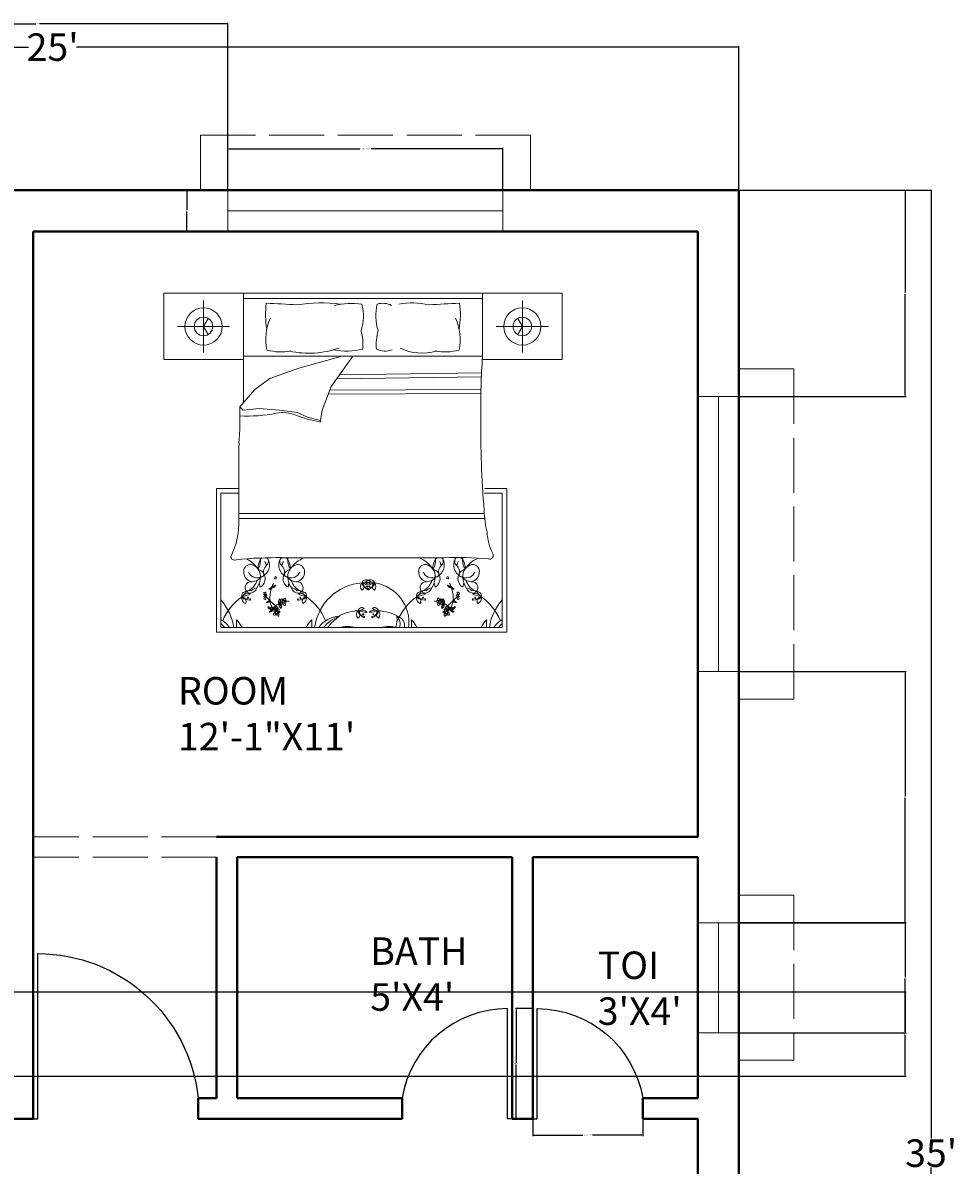
# Model space of a CAD drawing. Units: inches. Extents: x -22 to 362, y -469 to 42.
# Tile 6 of 6: x 158 to 362, y -207 to 42. Entities that reach past the tile are written whole.
import ezdxf

# ---------------------------------------------------------------- set-up
doc = ezdxf.new("R2010")
doc.units = ezdxf.units.IN
doc.header["$MEASUREMENT"] = 0
doc.linetypes.add('ACAD_ISO02W100', pattern=[15, 12, -3])
for name, color, linetype, lineweight in [('A-ANNO-DIMS', 2, 'Continuous', 18), ('A-AREA-IDEN', 7, 'Continuous', 25), ('A-DOOR', 3, 'Continuous', 25), ('A-FURN', 8, 'Continuous', 18), ('A-GLAZ', 4, 'Continuous', 20), ('A-ROOF-OVHD', 8, 'ACAD_ISO02W100', 18), ('A-WALL', 7, 'Continuous', 40), ('A-WALL-OVHD', 7, 'ACAD_ISO02W100', 18)]:
    doc.layers.add(name, color=color, linetype=linetype, lineweight=lineweight)
doc.styles.get("Standard").update_dxf_attribs({"font": 'arial.ttf'})
doc.dimstyles.get("Standard").update_dxf_attribs({"dimtxt": 0.18, "dimasz": 0.18, "dimexe": 0.18, "dimexo": 0.0625, "dimgap": 0.09, "dimtad": 0, "dimtih": 1, "dimtoh": 1, "dimdec": 0, "dimzin": 0, "dimdsep": 46, "dimlunit": 3, "dimtxsty": 'Standard', "dimcen": 0.09, "dimadec": 0, "dimazin": 0, "dimtfac": 1, "dimtdec": 0, "dimtofl": 0, "dimtmove": 0, "dimatfit": 3, "dimfxl": 1, "dimtolj": 1, "dimtzin": 0, "dimarcsym": 0})

# ---------------------------------------------------------------- blocks, each defined once
blk = doc.blocks.new('*D5')
at = {"layer": 'A-ANNO-DIMS', "color": 0, "lineweight": -2, "transparency": 16777216}
for p, q in [((15.01, 5.76), (15.01, 37.04)), ((15.19, 36.86), (159.53, 36.86)), ((314.33, 36.86), (169.99, 36.86)), ((314.51, 5.76), (314.51, 37.04))]:
    blk.add_line(p, q, dxfattribs=at)
at = {"layer": 'A-ANNO-DIMS', "color": 0, "transparency": 16777216}
for points in [[(15.19, 36.89), (15.19, 36.83), (15.01, 36.86)], [(314.33, 36.89), (314.33, 36.83), (314.51, 36.86)]]:
    blk.add_solid(points, dxfattribs=at)
at = {"layer": 'Defpoints', "color": 0, "transparency": 16777216}
for p in [(314.51, 36.86), (15.01, 5.69), (314.51, 5.69)]:
    blk.add_point(p, dxfattribs=at)
at = {"layer": 'A-ANNO-DIMS', "color": 0, "transparency": 16777216, "insert": (164.76, 36.86), "char_height": 6, "attachment_point": 5}
blk.add_mtext("\\A1;25'", dxfattribs=at)
blk = doc.blocks.new('*D6')
at = {"layer": 'A-ANNO-DIMS', "color": 0, "lineweight": -2, "transparency": 16777216}
for p, q in [((314.57, 5.69), (356.62, 5.69)), ((356.44, 5.51), (356.44, -201.15)), ((356.44, -414.13), (356.44, -207.46)), ((314.57, -414.31), (356.62, -414.31))]:
    blk.add_line(p, q, dxfattribs=at)
at = {"layer": 'A-ANNO-DIMS', "color": 0, "transparency": 16777216}
for points in [[(356.41, 5.51), (356.47, 5.51), (356.44, 5.69)], [(356.41, -414.13), (356.47, -414.13), (356.44, -414.31)]]:
    blk.add_solid(points, dxfattribs=at)
at = {"layer": 'Defpoints', "color": 0, "transparency": 16777216}
for p in [(314.51, 5.69), (314.51, -414.31), (356.44, -414.31)]:
    blk.add_point(p, dxfattribs=at)
at = {"layer": 'A-ANNO-DIMS', "color": 0, "transparency": 16777216, "insert": (356.44, -204.31), "char_height": 6, "attachment_point": 5}
blk.add_mtext("\\A1;35'", dxfattribs=at)
blk = doc.blocks.new('DOOR-SWING-36')
for p, q in [((-1, 0), (-1, 36)), ((0, 0), (-1, 0))]:
    blk.add_line(p, q)
blk.add_arc((-1, 0.81), 35.19, 90, 173.9744)
blk = doc.blocks.new('DOOR-SWING-24')
for p, q in [((-1, 0), (-1, 24)), ((0, 0), (-1, 0))]:
    blk.add_line(p, q)
blk.add_arc((-1, 0.69), 23.31, 90, 170.5843)
blk = doc.blocks.new('WIN-60-WALL9')
for p, q in [((0, 9), (60, 9)), ((0, 0), (0, 9)), ((60, 9), (60, 0)), ((0, 4.5), (60, 4.5)), ((60, 0), (0, 0))]:
    blk.add_line(p, q)
blk = doc.blocks.new('WINDOW-SHADE-72')
for p, q in [((12, 72), (0, 72)), ((12, 0), (12, 72)), ((0, 0), (12, 0))]:
    blk.add_line(p, q)
blk = doc.blocks.new('BED-DOUBLE-WITH-NIGHTSTANDS')
for p, q in [((0, 73.94), (86.94, 73.94)), ((8.69, 61.01), (8.69, 72.37)), ((17.39, 73.94), (17.39, 50.07)), ((69.55, 72.82), (17.39, 72.82)), ((78.25, 61.01), (78.25, 72.37)), ((14.37, 66.69), (3.01, 66.69)), ((72.57, 66.69), (83.93, 66.69)), ((17.39, 60.2), (69.55, 60.2)), ((29.46, 57.61), (38.94, 60.2)), ((41.27, 60.2), (36.51, 53.57)), ((23.13, 55.33), (29.46, 57.61)), ((19.78, 52.86), (23.13, 55.33)), ((69.29, 55.69), (37.72, 55.25)), ((69.32, 56.59), (38.37, 56.15)), ((16.61, 49.17), (19.78, 52.86)), ((36.51, 53.57), (34.57, 48.46)), ((69.24, 52.96), (36.23, 52.83)), ((69.24, 52.06), (35.89, 51.93)), ((17.31, 48.46), (16.61, 49.17)), ((20.84, 48.81), (17.31, 48.46)), ((25.24, 48.46), (20.84, 48.81)), ((29.11, 47.94), (25.24, 48.46)), ((31.4, 46.88), (29.11, 47.94)), ((34.57, 48.46), (34.22, 46.18)), ((34.22, 46.18), (31.4, 46.88)), ((11.48, 31.32), (16.39, 31.32)), ((11.48, 0), (11.48, 31.32)), ((16.39, 30.31), (12.48, 30.31)), ((12.48, 30.31), (12.48, 1.01)), ((73.85, 30.31), (70.02, 30.31)), ((70.04, 31.32), (74.86, 31.32)), ((73.85, 1.01), (73.85, 30.31)), ((74.86, 31.32), (74.86, 0)), ((69.95, 25.9), (16.39, 25.9)), ((70.03, 24.81), (16.39, 24.81)), ((61.12, 16.27), (25.82, 16.27)), ((21.05, 9.82), (20.86, 10.8)), ((27.13, 9.82), (27.32, 10.8)), ((59.21, 9.82), (59.02, 10.8)), ((65.28, 9.82), (65.48, 10.8)), ((74.86, 0), (11.48, 0)), ((12.48, 1.01), (73.85, 1.01))]:
    blk.add_line(p, q)
for points in [[(17.39, 59.45), (0, 59.45), (0, 73.94)], [(69.55, 73.94), (69.55, 59.45), (86.94, 59.45), (86.94, 73.94)], [(8.69, 66.69), (9.71, 68.45)], [(78.25, 66.69), (77.23, 68.45)], [(8.69, 66.69), (9.71, 64.94)], [(78.25, 66.69), (77.23, 64.94)]]:
    blk.add_lwpolyline(points)
for points in [[(22.38, 71.77, 0.074897), (22.49, 66.09, -0.472817)], [(43.06, 65.77, 0.14099), (43.24, 71.57, 0.235245)], [(46.78, 65.77, -0.14099), (46.6, 71.57, -0.235245)], [(64.56, 71.77, -0.074897), (64.45, 66.09, 0.472817)], [(16.43, 41.21, 0.001242), (16.39, 24.71, -0.127202), (14.64, 16.49)], [(69.92, 26.58, 0.056112), (70.55, 21.8, 0.095341), (71.78, 17.19)]]:
    blk.add_lwpolyline(points, format="xyb")
for centre, radius in [((8.69, 66.69), 4.06), ((78.25, 66.69), 4.06), ((8.69, 66.69), 2.03), ((78.25, 66.69), 2.03), ((26.07, 6.67), 0.221), ((60.26, 6.67), 0.221), ((24.62, 4.34), 0.221), ((61.71, 4.34), 0.221)]:
    blk.add_circle(centre, radius)
for centre, radius, start, end in [((70.3, 899.16), 828.77, 266.68521, 267.14978), ((34.29, 40.31), 31.53, 82.2196, 99.497), ((40.95, 56.24), 15.49, 81.5249, 103.96), ((47.79, 67.44), 4.3, 63.3437, 106.1026), ((54.24, 56.56), 15.28, 76.3427, 101.1841), ((16.64, 899.16), 828.77, 272.85022, 273.31479), ((33.46, 63.81), 11.21, 155.1316, 191.7583), ((53.48, 63.81), 11.21, 348.2417, 24.8684), ((32.81, 62.87), 10.65, 354.0129, 15.8293), ((57.02, 62.87), 10.65, 164.1707, 185.9871), ((25.48, 72.79), 11.65, 255.1039, 281.0369), ((31.62, 81.07), 20.21, 258.0397, 289.2615), ((39.8, 76.66), 15.33, 259.8617, 283.6238), ((48.38, 65.93), 4.61, 245.0183, 288.5407), ((56.43, 71.93), 11.07, 243.8761, 286.1746), ((61.46, 72.79), 11.65, 258.9631, 284.8961), ((225.41, 49.57), 156.22, 176.1, 180.9282), ((-63.11, 47.01), 79.74, 355.8294, 1.553), ((18.1, 79.95), 32.81, 267.4519, 281.3392), ((25.94, 40.84), 7.08, 66.2616, 101.3392), ((40.26, 79.03), 33.72, 250.1194, 259.3383), ((34.02, 46.1), 0.21, 268.8623, 19.7536), ((272.96, 43.89), 203.78, 179.1145, 184.8735), ((15.44, 16.54), 0.802, 183.98, 297.3412), ((24.78, -74.23), 90.51, 89.3433, 95.6887), ((15.1, 10.15), 6.58, 33.6671, 63.2997), ((23.92, 14.06), 3.35, 145.785, 184.7304), ((17.52, 15.63), 3.6, 328.8218, 9.1554), ((21.98, 15.31), 1.05, 120.0293, 142.325), ((20.31, 14.69), 2.77, 289.2822, 29.1751), ((19.89, 14.19), 2.5, 7.436, 29.9149), ((21.54, 15.52), 1.3, 311.5653, 23.8354), ((21.98, 15.31), 1.05, 44.4517, 63.558), ((27.87, 14.69), 2.77, 150.8249, 250.7178), ((26.64, 15.52), 1.3, 156.1646, 228.4347), ((26.2, 15.31), 1.05, 113.229, 135.5483), ((28.29, 14.19), 2.5, 150.0851, 172.564), ((26.2, 15.31), 1.05, 37.675, 66.7144), ((24.25, 14.06), 3.35, 355.2696, 34.215), ((30.66, 15.63), 3.6, 169.7133, 211.1782), ((33.07, 10.15), 6.58, 111.4941, 146.3329), ((53.26, 10.15), 6.58, 33.6671, 68.5059), ((62.08, 14.06), 3.35, 145.785, 184.7304), ((55.68, 15.63), 3.6, 328.8218, 10.2867), ((60.14, 15.31), 1.05, 113.2856, 142.325), ((58.46, 14.69), 2.77, 289.2822, 29.1751), ((58.05, 14.19), 2.5, 7.436, 29.9149), ((60.14, 15.31), 1.05, 44.4517, 66.7144), ((59.69, 15.52), 1.3, 311.5653, 23.8354), ((63.78, -68.29), 84.6, 85.2402, 91.8035), ((66.03, 14.69), 2.77, 150.8249, 250.7178), ((64.8, 15.52), 1.3, 156.1646, 228.4347), ((64.35, 15.31), 1.05, 106.6343, 135.5483), ((66.44, 14.19), 2.5, 150.0851, 172.564), ((64.35, 15.31), 1.05, 37.675, 72.5814), ((62.41, 14.06), 3.35, 355.2696, 34.215), ((68.82, 15.63), 3.6, 169.249, 211.1782), ((71.23, 10.15), 6.58, 113.6453, 146.3329), ((71.12, 16.75), 0.792, 246.5219, 33.8264), ((19.54, 13.1), 2.08, 174.9449, 262.8857), ((18.94, 13.31), 1.47, 84.4856, 181.0538), ((20.36, 13.89), 2.02, 201.5819, 291.4221), ((18.49, 12.22), 2.61, 355.2933, 76.921), ((19.97, 11.7), 2.16, 299.9085, 73.1337), ((21.34, 12.6), 0.54, 257.3041, 15.1471), ((23.58, 13.21), 1.78, 131.5653, 195.1471), ((24.59, 13.21), 1.78, 344.8529, 48.4347), ((28.2, 11.7), 2.16, 106.8663, 240.0915), ((26.84, 12.6), 0.54, 164.8529, 282.6959), ((29.69, 12.22), 2.61, 103.079, 184.7067), ((27.82, 13.89), 2.02, 248.5779, 338.4181), ((28.64, 13.1), 2.08, 277.1143, 5.0551), ((29.24, 13.31), 1.47, 358.9462, 95.5144), ((57.7, 13.1), 2.08, 174.9449, 262.8857), ((57.09, 13.31), 1.47, 84.4856, 181.0538), ((58.51, 13.89), 2.02, 201.5819, 291.4221), ((56.64, 12.22), 2.61, 355.2933, 76.921), ((58.13, 11.7), 2.16, 299.9085, 73.1337), ((59.5, 12.6), 0.54, 257.3041, 15.1471), ((61.74, 13.21), 1.78, 131.5653, 195.1471), ((62.75, 13.21), 1.78, 344.8529, 48.4347), ((66.36, 11.7), 2.16, 106.8663, 240.0915), ((64.99, 12.6), 0.54, 164.8529, 282.6959), ((67.85, 12.22), 2.61, 103.079, 184.7067), ((65.98, 13.89), 2.02, 248.5779, 338.4181), ((66.79, 13.1), 2.08, 277.1143, 5.0551), ((67.4, 13.31), 1.47, 358.9462, 95.5144), ((19.06, 9.75), 1.3, 80.264, 250.8688), ((16.47, 12.62), 4.1, 301.2614, 341.7045), ((19.18, 13.56), 2.53, 272.3591, 324.0401), ((16.44, 12.29), 4.67, 326.2883, 356.5076), ((23.92, 14.06), 3.35, 212.7011, 216.3445), ((30.36, 7.41), 7.2, 153.0032, 159.8941), ((23.87, 9.87), 0.177, 84.3784, 186.0543), ((23.52, 11.4), 1.4, 285.5129, 293.6099), ((23.37, 11.14), 1.37, 301.164, 321.5612), ((24.43, 9.82), 0.456, 87.3579, 140.4944), ((24.34, 11.79), 0.168, 102.7051, 280.4384), ((22.26, 11.38), 2.45, 324.6898, 333.4936), ((24.32, 11.89), 0.272, 280.4384, 100.4136), ((24.25, 14.06), 3.35, 323.6555, 327.2989), ((29, 13.56), 2.53, 215.9599, 267.6409), ((31.74, 12.29), 4.67, 183.4924, 213.7117), ((31.7, 12.62), 4.1, 198.2955, 238.7386), ((29.12, 9.75), 1.3, 289.1312, 99.736), ((44.15, -0.52), 11.35, 94.4623, 172.255), ((44.2, 9.95), 1.26, 137.7873, 219.1145), ((42.77, 9.99), 0.948, 298.5391, 58.3627), ((44.17, 10.53), 0.941, 63.0274, 163.8037), ((43.21, 12.73), 1.94, 271.4585, 315.3727), ((44, 9.16), 1.79, 45.5411, 114.3101), ((45.64, 18.38), 7.94, 252.593, 267.2582), ((44.19, 10.76), 0.929, 177.7585, 283.852), ((45.98, 11.73), 2.87, 198.9159, 238.011), ((45.23, 9.16), 1.79, 65.6899, 134.4589), ((43.59, 18.38), 7.94, 272.7418, 287.407), ((44.38, 9.98), 0.123, 283.852, 219.9245), ((45.07, 10.53), 0.941, 16.1963, 116.9726), ((46.02, 12.73), 1.94, 224.6273, 268.5415), ((44.84, 10.03), 0.074, 320.1909, 256.0209), ((43.25, 11.73), 2.87, 301.989, 341.0841), ((45.04, 10.76), 0.929, 256.148, 2.2415), ((46.47, 9.99), 0.948, 121.6373, 241.4609), ((45.04, 9.95), 1.26, 320.8855, 42.2127), ((44.72, 2.1), 8.79, 352.8636, 81.8197), ((57.22, 9.75), 1.3, 80.264, 250.8688), ((54.63, 12.62), 4.1, 301.2614, 341.7045), ((57.34, 13.56), 2.53, 272.3591, 324.0401), ((54.59, 12.29), 4.67, 326.2883, 356.5076), ((62.08, 14.06), 3.35, 212.7011, 216.3445), ((62.01, 11.89), 0.272, 79.5864, 259.5616), ((62.96, 11.14), 1.37, 218.4388, 238.836), ((61.9, 9.82), 0.456, 39.5056, 92.6421), ((64.08, 11.38), 2.45, 206.5064, 215.3102), ((62, 11.79), 0.168, 259.5616, 77.2949), ((62.82, 11.4), 1.4, 246.3901, 254.4871), ((55.97, 7.41), 7.2, 20.1059, 26.9968), ((62.46, 9.87), 0.177, 353.9457, 95.6216), ((62.41, 14.06), 3.35, 323.6555, 327.2989), ((67.16, 13.56), 2.53, 215.9599, 267.6409), ((69.9, 12.29), 4.67, 183.4924, 213.7117), ((69.86, 12.62), 4.1, 198.2955, 238.7386), ((67.27, 9.75), 1.3, 289.1312, 99.736), ((23.45, -1.64), 11.35, 124.3865, 158.5908), ((18.27, 7.46), 1.26, 167.7115, 249.0387), ((17.96, 7.95), 0.941, 92.9516, 193.728), ((16.03, 9.38), 1.94, 301.3827, 345.2969), ((18.5, 6.68), 1.79, 75.4653, 144.2343), ((15.32, 15.48), 7.94, 282.5173, 297.1824), ((17.01, 6.78), 0.948, 328.4633, 88.2869), ((18.93, 9.89), 2.87, 228.8402, 267.9352), ((17.86, 8.16), 0.929, 207.6827, 313.7762), ((18.79, 8.34), 0.8, 63.9755, 143.2681), ((18.42, 7.57), 0.123, 313.7762, 249.7183), ((18.75, 10.14), 1.63, 265.969, 344.3045), ((20.5, 7.98), 1.74, 96.1662, 141.5825), ((22.09, 8.33), 0.369, 101.5637, 142.6358), ((21.78, 7.99), 0.221, 273.2768, 86.7232), ((22.04, 8.2), 0.211, 91.1081, 181.8675), ((22.48, 8.06), 0.672, 203.4276, 227.6104), ((22.26, 7.77), 0.458, 80.3487, 133.6538), ((22.18, 8.15), 0.362, 229.7889, 317.6792), ((21.79, 8.62), 0.532, 288.7263, 352.5032), ((21.77, 7.38), 0.515, 355.053, 68.3618), ((22.18, 7.3), 0.725, 83.0852, 105.7171), ((22.15, 8.59), 0.171, 345.2356, 144.9248), ((17.16, 1.28), 8.25, 43.1541, 52.0459), ((22.31, 8.03), 0.191, 317.6792, 80.3487), ((23.38, 9.2), 0.456, 101.3256, 154.4621), ((22.72, 10.74), 1.37, 280.2588, 300.656), ((23.04, 11.84), 2.45, 268.3264, 277.1302), ((30.36, 7.41), 7.2, 163.5842, 183.8277), ((22.42, 10.74), 1.4, 308.2101, 316.3071), ((23.28, 9.82), 0.417, 278.3432, 4.2869), ((23.05, 10.19), 0.729, 300.656, 332.6341), ((23.6, 9.71), 0.177, 55.7657, 157.4417), ((23.71, 10.58), 0.729, 269.1859, 301.164), ((23.92, 10.21), 0.417, 237.5332, 323.4768), ((27.67, 7.98), 1.74, 38.4175, 83.8338), ((29.43, 10.14), 1.63, 195.6955, 274.031), ((29.38, 8.34), 0.8, 36.7319, 116.0245), ((29.68, 6.68), 1.79, 35.7657, 104.5347), ((32.86, 15.48), 7.94, 242.8176, 257.4827), ((29.24, 9.89), 2.87, 272.0648, 311.1598), ((30.31, 8.16), 0.929, 226.2238, 332.3173), ((29.77, 7.62), 0.074, 290.2667, 226.2271), ((31.16, 6.78), 0.948, 91.7131, 211.5367), ((30.22, 7.95), 0.941, 346.272, 87.0484), ((32.14, 9.38), 1.94, 194.7031, 238.6173), ((29.9, 7.46), 1.26, 290.9613, 12.2885), ((24.72, -1.64), 11.35, 21.4092, 55.6135), ((44.53, 9.41), 0.141, 238.011, 71.5592), ((44.56, 9.48), 0.0685, 71.5592, 188.0167), ((44.7, 9.41), 0.141, 108.4408, 301.989), ((44.68, 9.48), 0.0685, 351.9833, 108.4408), ((61.61, -1.64), 11.35, 124.3865, 158.5908), ((56.11, 7.95), 0.941, 92.9516, 193.728), ((56.43, 7.46), 1.26, 167.7115, 249.0387), ((54.19, 9.38), 1.94, 301.3827, 345.2969), ((56.66, 6.68), 1.79, 75.4653, 144.2343), ((53.48, 15.48), 7.94, 282.5173, 297.1824), ((56.02, 8.16), 0.929, 207.6827, 313.7762), ((57.09, 9.89), 2.87, 228.8402, 267.9352), ((55.17, 6.78), 0.948, 328.4633, 88.2869), ((56.95, 8.34), 0.8, 63.9755, 143.2681), ((56.58, 7.57), 0.123, 313.7762, 249.7183), ((56.91, 10.14), 1.63, 265.969, 344.3045), ((58.66, 7.98), 1.74, 96.1662, 141.5825), ((62.41, 10.21), 0.417, 216.5232, 302.4668), ((62.63, 10.58), 0.729, 238.836, 270.8141), ((62.74, 9.71), 0.177, 22.5583, 124.2343), ((63.05, 9.82), 0.417, 175.7131, 261.6568), ((63.28, 10.19), 0.729, 207.3659, 239.344), ((55.97, 7.41), 7.2, 356.1723, 16.4158), ((63.91, 10.74), 1.4, 223.6929, 231.7899), ((63.61, 10.74), 1.37, 239.344, 259.7412), ((63.3, 11.84), 2.45, 262.8698, 271.6736), ((62.96, 9.2), 0.456, 25.5379, 78.6744), ((69.18, 1.28), 8.25, 127.9541, 136.8459), ((64.03, 8.03), 0.191, 99.6513, 222.3208), ((64.15, 8.15), 0.362, 222.3208, 310.2111), ((64.07, 7.77), 0.458, 46.3462, 99.6513), ((64.18, 8.59), 0.171, 35.0752, 194.7644), ((64.54, 8.62), 0.532, 187.4968, 251.2737), ((64.56, 7.38), 0.515, 111.6382, 184.947), ((64.16, 7.3), 0.725, 74.2829, 96.9148), ((64.29, 8.2), 0.211, 358.1325, 88.8919), ((63.86, 8.06), 0.672, 312.3896, 336.5724), ((64.25, 8.33), 0.369, 37.3642, 78.4363), ((64.55, 7.99), 0.221, 93.2768, 266.7232), ((67.59, 10.14), 1.63, 195.6955, 274.031), ((65.83, 7.98), 1.74, 38.4175, 83.8338), ((67.54, 8.34), 0.8, 36.7319, 116.0245), ((67.84, 6.68), 1.79, 35.7657, 104.5347), ((71.01, 15.48), 7.94, 242.8176, 257.4827), ((67.4, 9.89), 2.87, 272.0648, 311.1598), ((68.47, 8.16), 0.929, 226.2238, 332.3173), ((67.93, 7.62), 0.074, 290.2667, 226.2271), ((69.32, 6.78), 0.948, 91.7131, 211.5367), ((70.3, 9.38), 1.94, 194.7031, 238.6173), ((68.38, 7.95), 0.941, 346.272, 87.0484), ((68.06, 7.46), 1.26, 290.9613, 12.2885), ((62.88, -1.64), 11.35, 21.4092, 55.6135), ((4.03, -0.52), 11.35, 7.745, 41.8856), ((18.82, 7.23), 0.0685, 101.4834, 217.9409), ((18.83, 7.16), 0.141, 267.9352, 101.4834), ((22.08, 7.58), 0.366, 217.7621, 259.0403), ((22.12, 7.35), 0.17, 232.4737, 355.053), ((22.86, 6.27), 0.456, 101.3256, 154.4621), ((22.2, 7.82), 1.37, 280.2588, 300.656), ((22.52, 8.92), 2.45, 268.3264, 277.1302), ((21.91, 7.82), 1.4, 308.2101, 316.3071), ((23.01, 5.47), 0.247, 146.8636, 236.9021), ((26.5, 10.92), 6.47, 235.1882, 238.8844), ((23.44, 5.83), 0.669, 199.4799, 267.6828), ((22.76, 6.9), 0.417, 278.3432, 4.2869), ((23.36, 5.57), 0.576, 212.8155, 277.3992), ((22.53, 7.26), 0.729, 300.656, 332.6341), ((23.08, 6.78), 0.177, 55.7657, 157.4417), ((23.29, 5.6), 0.256, 238.8844, 314.2646), ((26.78, 7.23), 3.61, 184.756, 209.2041), ((31.97, 14.91), 11.88, 222.2412, 232.1744), ((23.23, 5.02), 0.576, 280.3057, 17.1958), ((23.18, 4.96), 0.256, 306.3746, 21.7548), ((23.6, 5.13), 0.193, 19.3605, 201.7548), ((23.6, 5.27), 0.193, 311.8703, 134.2646), ((27.23, 3.52), 3.86, 153.7819, 158.2913), ((24.16, 6.15), 1.01, 247.2305, 319.0635), ((23.83, 5.81), 0.594, 264.4544, 310.6188), ((26.78, 7.23), 3.61, 214.0033, 222.4917), ((24.27, 5.57), 0.613, 218.3208, 298.8162), ((27.15, 2.43), 4.33, 120.544, 139.818), ((24.68, 4.82), 0.714, 70.0041, 130.6188), ((24.22, 5.69), 0.733, 297.7043, 344.3516), ((24.93, 4.68), 0.369, 101.5637, 176.365), ((25, 4.94), 0.171, 345.2356, 144.9248), ((24.38, 7), 1.01, 304.5369, 16.3699), ((24.92, 6.78), 0.613, 272.8499, 356.1226), ((24.48, 6.54), 0.594, 321.7607, 7.9252), ((24.61, 5.68), 0.594, 8.7227, 54.8872), ((24.64, 5.21), 1.01, 0.278, 72.111), ((25.78, 6.72), 0.714, 127.3105, 187.9252), ((25.09, 5.58), 0.613, 20.5253, 88.5375), ((25.9, 5.88), 0.714, 188.7227, 249.3375), ((24.8, 6.8), 0.733, 355.0106, 41.658), ((25.61, 6.26), 0.219, 148.0499, 225.6268), ((27.15, 2.43), 4.33, 113.0501, 113.8477), ((26.01, 6), 0.698, 104.7558, 148.0499), ((25.62, 6.5), 0.437, 247.4086, 351.4386), ((25.83, 6.98), 0.302, 126.1046, 271.4281), ((25.8, 7.06), 0.217, 353.7526, 131.7054), ((24.99, 5.52), 0.733, 334.9899, 21.6373), ((25.75, 6.48), 0.147, 262.906, 7.132), ((25.59, 6.8), 0.305, 0.0645, 61.1507), ((25.66, 7.06), 0.348, 311.8413, 355.7877), ((26.38, 7.01), 0.369, 101.5637, 176.365), ((26.37, 6.26), 0.366, 151.2196, 259.0403), ((26.33, 6.88), 0.211, 91.1081, 181.8675), ((26.77, 6.75), 0.672, 203.4276, 227.6104), ((26.56, 6.46), 0.458, 80.3487, 133.6538), ((26.47, 6.83), 0.362, 229.7889, 317.6792), ((26.08, 7.3), 0.532, 288.7263, 352.5032), ((26.07, 6.07), 0.515, 355.053, 68.3618), ((26.47, 5.98), 0.725, 83.0852, 105.7171), ((26.45, 7.28), 0.171, 345.2356, 144.9248), ((26.41, 6.04), 0.17, 232.4737, 355.053), ((26.6, 6.72), 0.191, 317.6792, 80.3487), ((27.15, 2.43), 4.33, 87.1071, 94.7585), ((29.34, 7.16), 0.141, 78.5166, 272.0648), ((29.36, 7.23), 0.0685, 322.0591, 78.5166), ((43.3, 4.45), 0.941, 63.0274, 163.8037), ((42.34, 6.65), 1.94, 271.4585, 315.3727), ((45.93, 4.45), 0.941, 16.1963, 116.9726), ((46.89, 6.65), 1.94, 224.6273, 268.5415), ((56.98, 7.23), 0.0685, 101.4834, 217.9409), ((56.99, 7.16), 0.141, 267.9352, 101.4834), ((59.19, 2.43), 4.33, 85.2415, 92.8929), ((59.73, 6.72), 0.191, 99.6513, 222.3208), ((59.86, 6.83), 0.362, 222.3208, 310.2111), ((59.78, 6.46), 0.458, 46.3462, 99.6513), ((59.89, 7.28), 0.171, 35.0752, 194.7644), ((60.25, 7.3), 0.532, 187.4968, 251.2737), ((60.27, 6.07), 0.515, 111.6382, 184.947), ((59.93, 6.04), 0.17, 184.947, 307.5263), ((59.87, 5.98), 0.725, 74.2829, 96.9148), ((60, 6.88), 0.211, 358.1325, 88.8919), ((59.56, 6.75), 0.672, 312.3896, 336.5724), ((59.95, 7.01), 0.369, 3.635, 78.4363), ((59.96, 6.26), 0.366, 280.9597, 28.7804), ((60.71, 6.5), 0.437, 188.5614, 292.5914), ((60.54, 7.06), 0.217, 48.2946, 186.2474), ((60.67, 7.06), 0.348, 184.2123, 228.1587), ((60.74, 6.8), 0.305, 118.8493, 179.9355), ((60.59, 6.48), 0.147, 172.868, 277.094), ((60.51, 6.98), 0.302, 268.5719, 53.8954), ((60.32, 6), 0.698, 31.9501, 75.2442), ((61.35, 5.52), 0.733, 158.3627, 205.0101), ((61.24, 5.58), 0.613, 91.4625, 159.4747), ((61.69, 5.21), 1.01, 107.889, 179.722), ((60.43, 5.88), 0.714, 290.6625, 351.2773), ((61.54, 6.8), 0.733, 138.342, 184.9894), ((61.42, 6.78), 0.613, 183.8774, 267.1501), ((59.19, 2.43), 4.33, 66.1523, 66.9499), ((60.73, 6.26), 0.219, 314.3732, 31.9501), ((61.96, 7), 1.01, 163.6301, 235.4631), ((60.55, 6.72), 0.714, 352.0748, 52.6895), ((61.73, 5.68), 0.594, 125.1128, 171.2773), ((61.34, 4.94), 0.171, 35.0752, 194.7644), ((61.85, 6.54), 0.594, 172.0748, 218.2393), ((59.19, 2.43), 4.33, 40.182, 59.456), ((61.65, 4.82), 0.714, 49.3812, 109.9959), ((62.17, 6.15), 1.01, 220.9365, 292.7695), ((62.11, 5.69), 0.733, 195.6484, 242.2957), ((61.4, 4.68), 0.369, 3.635, 78.4363), ((54.36, 14.91), 11.88, 307.8256, 317.7588), ((62.07, 5.57), 0.613, 241.1838, 321.6792), ((62.5, 5.81), 0.594, 229.3812, 275.5456), ((59.56, 7.23), 3.61, 317.5083, 325.9967), ((63.1, 5.02), 0.576, 162.8042, 259.6943), ((62.73, 5.27), 0.193, 45.7354, 228.1297), ((62.73, 5.13), 0.193, 338.2452, 160.6395), ((59.1, 3.52), 3.86, 21.7087, 26.2181), ((59.56, 7.23), 3.61, 330.7959, 355.244), ((63.04, 5.6), 0.256, 225.7354, 301.1156), ((63.15, 4.96), 0.256, 158.2452, 233.6254), ((62.97, 5.57), 0.576, 262.6008, 327.1845), ((62.9, 5.83), 0.669, 272.3172, 340.5201), ((63.25, 6.78), 0.177, 22.5583, 124.2343), ((63.57, 6.9), 0.417, 175.7131, 261.6568), ((63.8, 7.26), 0.729, 207.3659, 239.344), ((59.83, 10.92), 6.47, 301.1156, 304.8118), ((64.43, 7.82), 1.4, 223.6929, 231.7899), ((64.13, 7.82), 1.37, 239.344, 259.7412), ((63.32, 5.47), 0.247, 303.0979, 33.1364), ((63.81, 8.92), 2.45, 262.8698, 271.6736), ((63.47, 6.27), 0.456, 25.5379, 78.6744), ((64.22, 7.35), 0.17, 184.947, 307.5263), ((64.25, 7.58), 0.366, 280.9597, 322.2379), ((67.5, 7.16), 0.141, 78.5166, 272.0648), ((67.51, 7.23), 0.0685, 322.0591, 78.5166), ((82.3, -0.52), 11.35, 138.1144, 172.255), ((9.73, -2.04), 5.53, 33.4617, 60.1116), ((12.82, -0.76), 4.62, 22.5547, 48.9546), ((0.18, 1.72), 15.71, 357.4081, 3.6519), ((23.03, 5.19), 0.669, 266.9701, 338.2913), ((19.5, 9.97), 6.47, 302.6784, 306.3746), ((23.2, 4.66), 0.247, 214.3538, 304.3923), ((24.16, 3.92), 0.219, 148.0499, 225.6268), ((24.57, 3.67), 0.698, 104.7558, 148.0499), ((24.17, 4.17), 0.437, 247.4086, 351.4386), ((24.38, 4.65), 0.302, 126.1046, 271.4281), ((24.35, 4.73), 0.217, 353.7526, 131.7054), ((24.3, 4.15), 0.147, 262.906, 7.132), ((24.14, 4.47), 0.305, 0.0645, 61.1507), ((24.22, 4.73), 0.348, 311.8413, 355.7877), ((24.93, 3.93), 0.366, 151.2196, 259.0403), ((24.88, 4.55), 0.211, 91.1081, 181.8675), ((25.32, 4.41), 0.672, 203.4276, 227.6104), ((25.11, 4.12), 0.458, 80.3487, 133.6538), ((25.03, 4.5), 0.362, 229.7889, 317.6792), ((24.63, 4.97), 0.532, 288.7263, 352.5032), ((24.62, 3.73), 0.515, 355.053, 68.3618), ((25.02, 3.65), 0.725, 83.0852, 105.7171), ((24.96, 3.7), 0.17, 232.4737, 355.053), ((25.15, 4.39), 0.191, 317.6792, 80.3487), ((35.35, -0.76), 4.62, 131.0454, 157.4453), ((48, 1.72), 15.71, 176.3481, 182.5919), ((38.45, -2.04), 5.53, 91.272, 146.5383), ((40.44, -3.07), 6.89, 107.8504, 143.6964), ((44.06, -5.01), 10.25, 124.0123, 144.053), ((43.28, -6.6), 11.35, 94.4623, 117.4146), ((43.33, 3.87), 1.26, 137.7873, 219.1145), ((41.9, 3.91), 0.948, 298.5391, 58.3627), ((43.13, 3.08), 1.79, 45.5411, 114.3101), ((45.11, 5.65), 2.87, 198.9159, 238.011), ((44.77, 12.29), 7.94, 252.593, 267.2582), ((43.32, 4.68), 0.929, 177.7585, 283.852), ((43.51, 3.9), 0.123, 283.852, 219.9245), ((43.66, 3.33), 0.141, 238.011, 71.5592), ((43.69, 3.4), 0.0685, 71.5592, 188.0167), ((46.1, 3.08), 1.79, 65.6899, 134.4589), ((44.46, 12.29), 7.94, 272.7418, 287.407), ((45.57, 3.33), 0.141, 108.4408, 301.989), ((45.55, 3.4), 0.0685, 351.9833, 108.4408), ((45.71, 3.94), 0.074, 320.1909, 256.0209), ((44.12, 5.65), 2.87, 301.989, 341.0841), ((45.91, 4.68), 0.929, 256.148, 2.2415), ((47.34, 3.91), 0.948, 121.6373, 241.4609), ((45.91, 3.87), 1.26, 320.8855, 42.2127), ((45.95, -6.6), 11.35, 62.5854, 85.5377), ((45.85, 2.9), 5.08, 338.117, 6.6195), ((50.52, 1.49), 2.04, 346.3898, 79.0739), ((48.99, 1.77), 2.58, 342.8609, 41.9049), ((38.34, 1.72), 15.71, 357.4081, 3.6519), ((50.98, -0.76), 4.62, 22.5547, 48.9546), ((61.18, 4.39), 0.191, 99.6513, 222.3208), ((61.31, 4.5), 0.362, 222.3208, 310.2111), ((61.23, 4.12), 0.458, 46.3462, 99.6513), ((61.7, 4.97), 0.532, 187.4968, 251.2737), ((61.72, 3.73), 0.515, 111.6382, 184.947), ((61.37, 3.7), 0.17, 184.947, 307.5263), ((61.31, 3.65), 0.725, 74.2829, 96.9148), ((61.45, 4.55), 0.211, 358.1325, 88.8919), ((61.01, 4.41), 0.672, 312.3896, 336.5724), ((61.41, 3.93), 0.366, 280.9597, 28.7804), ((62.16, 4.17), 0.437, 188.5614, 292.5914), ((61.99, 4.73), 0.217, 48.2946, 186.2474), ((62.12, 4.73), 0.348, 184.2123, 228.1587), ((62.19, 4.47), 0.305, 118.8493, 179.9355), ((62.04, 4.15), 0.147, 172.868, 277.094), ((61.95, 4.65), 0.302, 268.5719, 53.8954), ((61.77, 3.67), 0.698, 31.9501, 75.2442), ((62.17, 3.92), 0.219, 314.3732, 31.9501), ((63.31, 5.19), 0.669, 201.7087, 273.0299), ((66.83, 9.97), 6.47, 233.6254, 237.3216), ((63.14, 4.66), 0.247, 235.6077, 325.6462), ((73.51, -0.76), 4.62, 131.0454, 157.4453), ((86.15, 1.72), 15.71, 176.3481, 182.5919), ((76.61, -2.04), 5.53, 119.8884, 146.5383), ((7.74, -3.07), 6.89, 36.3036, 46.4814), ((40.1, -4.96), 6.24, 73.5431, 107.0202), ((42.58, -8.18), 9.23, 94.3787, 95.6357), ((47.44, -14.5), 16.5, 109.7217, 109.9028), ((49.13, -4.96), 6.24, 72.9798, 106.4569), ((46.66, -8.18), 9.23, 84.3643, 85.6213), ((41.79, -14.5), 16.5, 70.0972, 70.2783), ((78.6, -3.07), 6.89, 133.5186, 143.6964)]:
    blk.add_arc(centre, radius, start, end)
blk = doc.blocks.new('*D14')
at = {"layer": 'A-ANNO-DIMS', "color": 0, "lineweight": -2, "transparency": 16777216}
for p, q in [((203.01, 5.76), (203.01, 14.87)), ((203.19, 14.69), (231.78, 14.69)), ((262.83, 14.69), (234.24, 14.69)), ((263.01, 5.76), (263.01, 14.87))]:
    blk.add_line(p, q, dxfattribs=at)
at = {"layer": 'A-ANNO-DIMS', "color": 0, "transparency": 16777216}
for points in [[(203.19, 14.72), (203.19, 14.66), (203.01, 14.69)], [(262.83, 14.72), (262.83, 14.66), (263.01, 14.69)]]:
    blk.add_solid(points, dxfattribs=at)
at = {"layer": 'Defpoints', "color": 0, "transparency": 16777216}
for p in [(203.01, 14.69), (203.01, 5.69), (263.01, 5.69)]:
    blk.add_point(p, dxfattribs=at)
at = {"layer": 'A-ANNO-DIMS', "color": 0, "transparency": 16777216, "insert": (233.01, 14.69), "char_height": 0.18, "attachment_point": 5}
blk.add_mtext('\\A1;WINDOW 5\'-0" TYP.', dxfattribs=at)
blk = doc.blocks.new('*D15')
at = {"layer": 'A-ANNO-DIMS', "color": 0, "lineweight": -2, "transparency": 16777216}
for p, q in [((202.95, 5.69), (193.83, 5.69)), ((194.01, 5.51), (194.01, 1.38)), ((194.01, -3.13), (194.01, 1.01)), ((202.95, -3.31), (193.83, -3.31))]:
    blk.add_line(p, q, dxfattribs=at)
at = {"layer": 'A-ANNO-DIMS', "color": 0, "transparency": 16777216}
for points in [[(193.98, 5.51), (194.04, 5.51), (194.01, 5.69)], [(193.98, -3.13), (194.04, -3.13), (194.01, -3.31)]]:
    blk.add_solid(points, dxfattribs=at)
at = {"layer": 'Defpoints', "color": 0, "transparency": 16777216}
for p in [(203.01, 5.69), (194.01, -3.31), (203.01, -3.31)]:
    blk.add_point(p, dxfattribs=at)
at = {"layer": 'A-ANNO-DIMS', "color": 0, "transparency": 16777216, "insert": (194.01, 1.19), "char_height": 0.18, "attachment_point": 5}
blk.add_mtext('\\A1;0\'-9" TYP.', dxfattribs=at)
blk = doc.blocks.new('*D20')
at = {"layer": 'A-ANNO-DIMS', "color": 0, "lineweight": -2, "transparency": 16777216}
for p, q in [((269.51, -196.87), (269.51, -200.59)), ((293.51, -196.87), (293.51, -200.59)), ((269.69, -200.41), (280.46, -200.41)), ((293.33, -200.41), (282.56, -200.41))]:
    blk.add_line(p, q, dxfattribs=at)
at = {"layer": 'A-ANNO-DIMS', "color": 0, "transparency": 16777216}
for points in [[(269.69, -200.38), (269.69, -200.44), (269.51, -200.41)], [(293.33, -200.38), (293.33, -200.44), (293.51, -200.41)]]:
    blk.add_solid(points, dxfattribs=at)
at = {"layer": 'Defpoints', "color": 0, "transparency": 16777216}
for p in [(269.51, -196.81), (293.51, -196.81), (269.51, -200.41)]:
    blk.add_point(p, dxfattribs=at)
at = {"layer": 'A-ANNO-DIMS', "color": 0, "transparency": 16777216, "insert": (281.51, -200.41), "char_height": 0.18, "attachment_point": 5}
blk.add_mtext('\\A1;DOOR 2\'-0" TYP.', dxfattribs=at)
blk = doc.blocks.new('*D21')
at = {"layer": 'A-ANNO-DIMS', "color": 0, "lineweight": -2, "transparency": 16777216}
for p, q in [((269.45, -172.81), (265.73, -172.81)), ((265.91, -172.99), (265.91, -184.62)), ((265.91, -196.63), (265.91, -184.99)), ((269.45, -196.81), (265.73, -196.81))]:
    blk.add_line(p, q, dxfattribs=at)
at = {"layer": 'A-ANNO-DIMS', "color": 0, "transparency": 16777216}
for points in [[(265.88, -172.99), (265.94, -172.99), (265.91, -172.81)], [(265.88, -196.63), (265.94, -196.63), (265.91, -196.81)]]:
    blk.add_solid(points, dxfattribs=at)
at = {"layer": 'Defpoints', "color": 0, "transparency": 16777216}
for p in [(265.91, -172.81), (269.51, -172.81), (269.51, -196.81)]:
    blk.add_point(p, dxfattribs=at)
at = {"layer": 'A-ANNO-DIMS', "color": 0, "transparency": 16777216, "insert": (265.91, -184.81), "char_height": 0.18, "attachment_point": 5}
blk.add_mtext('\\A1;2\'-0" TYP.', dxfattribs=at)
blk = doc.blocks.new('*D33')
at = {"layer": 'A-ANNO-DIMS', "color": 0, "lineweight": -2, "transparency": 16777216}
for p, q in [((120.01, 5.76), (120.01, 42.15)), ((120.19, 41.97), (161.11, 41.97)), ((202.83, 41.97), (161.91, 41.97)), ((203.01, 5.76), (203.01, 42.15))]:
    blk.add_line(p, q, dxfattribs=at)
at = {"layer": 'A-ANNO-DIMS', "color": 0, "transparency": 16777216}
for points in [[(120.19, 42), (120.19, 41.94), (120.01, 41.97)], [(202.83, 42), (202.83, 41.94), (203.01, 41.97)]]:
    blk.add_solid(points, dxfattribs=at)
at = {"layer": 'Defpoints', "color": 0, "transparency": 16777216}
for p in [(203.01, 41.97), (120.01, 5.69), (203.01, 5.69)]:
    blk.add_point(p, dxfattribs=at)
at = {"layer": 'A-ANNO-DIMS', "color": 0, "transparency": 16777216, "insert": (161.51, 41.97), "char_height": 0.18, "attachment_point": 5}
blk.add_mtext('\\A1;6\'-11"', dxfattribs=at)
blk = doc.blocks.new('*D38')
at = {"layer": 'A-ANNO-DIMS', "color": 0, "lineweight": -2, "transparency": 16777216}
for p, q in [((314.57, 5.69), (350.97, 5.69)), ((350.79, 5.51), (350.79, -16.62)), ((350.79, -39.13), (350.79, -16.99)), ((314.57, -39.31), (350.97, -39.31))]:
    blk.add_line(p, q, dxfattribs=at)
at = {"layer": 'A-ANNO-DIMS', "color": 0, "transparency": 16777216}
for points in [[(350.76, 5.51), (350.82, 5.51), (350.79, 5.69)], [(350.76, -39.13), (350.82, -39.13), (350.79, -39.31)]]:
    blk.add_solid(points, dxfattribs=at)
at = {"layer": 'Defpoints', "color": 0, "transparency": 16777216}
for p in [(314.51, 5.69), (314.51, -39.31), (350.79, -39.31)]:
    blk.add_point(p, dxfattribs=at)
at = {"layer": 'A-ANNO-DIMS', "color": 0, "transparency": 16777216, "insert": (350.79, -16.81), "char_height": 0.18, "attachment_point": 5}
blk.add_mtext('\\A1;3\'-9"', dxfattribs=at)
blk = doc.blocks.new('*D39')
at = {"layer": 'A-ANNO-DIMS', "color": 0, "lineweight": -2, "transparency": 16777216}
for p, q in [((314.573294, -99.306594), (350.970794, -99.306594)), ((350.790794, -99.486594), (350.790794, -126.501594)), ((350.790794, -153.876594), (350.790794, -126.861594)), ((314.573294, -154.056594), (350.970794, -154.056594))]:
    blk.add_line(p, q, dxfattribs=at)
at = {"layer": 'A-ANNO-DIMS', "color": 0, "transparency": 16777216}
for points in [[(350.760794, -99.486594), (350.820794, -99.486594), (350.790794, -99.306594)], [(350.760794, -153.876594), (350.820794, -153.876594), (350.790794, -154.056594)]]:
    blk.add_solid(points, dxfattribs=at)
at = {"layer": 'Defpoints', "color": 0, "transparency": 16777216}
for p in [(314.510794, -99.306594), (314.510794, -154.056594), (350.790794, -154.056594)]:
    blk.add_point(p, dxfattribs=at)
at = {"layer": 'A-ANNO-DIMS', "color": 0, "transparency": 16777216, "insert": (350.790794, -126.681594), "char_height": 0.18, "attachment_point": 5}
blk.add_mtext('\\A1;4\'-7"', dxfattribs=at)
blk = doc.blocks.new('*D40')
at = {"layer": 'A-ANNO-DIMS', "color": 0, "lineweight": -2, "transparency": 16777216}
for p, q in [((314.57, -154.06), (350.97, -154.06)), ((350.79, -154.24), (350.79, -165.87)), ((350.79, -177.88), (350.79, -166.24)), ((314.57, -178.06), (350.97, -178.06))]:
    blk.add_line(p, q, dxfattribs=at)
at = {"layer": 'A-ANNO-DIMS', "color": 0, "transparency": 16777216}
for points in [[(350.76, -154.24), (350.82, -154.24), (350.79, -154.06)], [(350.76, -177.88), (350.82, -177.88), (350.79, -178.06)]]:
    blk.add_solid(points, dxfattribs=at)
at = {"layer": 'Defpoints', "color": 0, "transparency": 16777216}
for p in [(314.51, -154.06), (314.51, -178.06), (350.79, -178.06)]:
    blk.add_point(p, dxfattribs=at)
at = {"layer": 'A-ANNO-DIMS', "color": 0, "transparency": 16777216, "insert": (350.79, -166.06), "char_height": 0.18, "attachment_point": 5}
blk.add_mtext('\\A1;2\'-0"', dxfattribs=at)
blk = doc.blocks.new('*D50')
at = {"layer": 'A-ANNO-DIMS', "color": 0, "lineweight": -2, "transparency": 16777216}
for p, q in [((92.59, -169.15), (350.97, -169.15)), ((350.79, -169.33), (350.79, -178.14)), ((350.79, -187.32), (350.79, -178.51)), ((92.59, -187.5), (350.97, -187.5))]:
    blk.add_line(p, q, dxfattribs=at)
at = {"layer": 'A-ANNO-DIMS', "color": 0, "transparency": 16777216}
for points in [[(350.76, -169.33), (350.82, -169.33), (350.79, -169.15)], [(350.76, -187.32), (350.82, -187.32), (350.79, -187.5)]]:
    blk.add_solid(points, dxfattribs=at)
at = {"layer": 'Defpoints', "color": 0, "transparency": 16777216}
for p in [(92.53, -169.15), (92.53, -187.5), (350.79, -187.5)]:
    blk.add_point(p, dxfattribs=at)
at = {"layer": 'A-ANNO-DIMS', "color": 0, "transparency": 16777216, "insert": (350.79, -178.33), "char_height": 0.18, "attachment_point": 5}
blk.add_mtext('\\A1;1\'-6 1/2"', dxfattribs=at)

msp = doc.modelspace()

# ---------------------------------------------------------------- linework, layer by layer
at = {"layer": 'A-GLAZ'}
for p, q in [((305.51, -154.06), (305.51, -178.06)), ((314.51, -154.06), (305.51, -154.06)), ((310.01, -154.06), (310.01, -178.06)), ((314.51, -178.06), (314.51, -154.06)), ((305.51, -178.06), (314.51, -178.06))]:
    msp.add_line(p, q, dxfattribs=at)
at = {"layer": 'A-ROOF-OVHD'}
for p, q in [((314.51, -148.06), (326.51, -148.06)), ((326.51, -148.06), (326.51, -184.06)), ((326.51, -184.06), (314.51, -184.06))]:
    msp.add_line(p, q, dxfattribs=at)
at = {"layer": 'A-WALL'}
for p, q in [((15.01, 5.69), (314.51, 5.69)), ((314.51, 5.69), (314.51, -414.31)), ((160.51, -3.31), (160.51, -196.81)), ((160.51, -3.31), (305.51, -3.31)), ((305.51, -3.31), (305.51, -135.31)), ((200.51, -135.31), (305.51, -135.31)), ((200.51, -139.81), (200.51, -192.31)), ((205.01, -139.81), (265.01, -139.81)), ((205.01, -139.81), (205.01, -192.31)), ((265.01, -139.81), (265.01, -192.31)), ((269.51, -139.81), (269.51, -192.31)), ((269.51, -139.81), (305.51, -139.81)), ((305.51, -139.81), (305.51, -192.31)), ((196.51, -192.31), (200.51, -192.31)), ((196.51, -192.31), (196.51, -196.81)), ((205.01, -192.31), (241.01, -192.31)), ((241.01, -192.31), (241.01, -196.81)), ((265.01, -192.31), (265.01, -196.81)), ((269.51, -192.31), (269.51, -196.81)), ((293.51, -192.31), (305.51, -192.31)), ((293.51, -192.31), (293.51, -196.81)), ((156.01, -196.81), (160.51, -196.81)), ((196.51, -196.81), (241.01, -196.81)), ((265.01, -196.81), (269.51, -196.81)), ((293.51, -196.81), (305.51, -196.81)), ((305.51, -196.81), (305.51, -321.31))]:
    msp.add_line(p, q, dxfattribs=at)
at = {"layer": 'A-WALL-OVHD'}
for p, q in [((200.51, -135.31), (160.51, -135.31)), ((200.51, -139.81), (160.51, -139.81))]:
    msp.add_line(p, q, dxfattribs=at)

# ---------------------------------------------------------------- block references
at = {"layer": 'A-DOOR', "extrusion": (0, 0, -1), "zscale": -1}
for name, p in [('DOOR-SWING-36', (-160.51, -196.81)), ('DOOR-SWING-24', (-269.51, -196.81))]:
    msp.add_blockref(name, p, dxfattribs=at)
at = {"layer": 'A-DOOR'}
msp.add_blockref('DOOR-SWING-24', (265.01, -196.81), dxfattribs=at)
at = {"layer": 'A-FURN'}
msp.add_blockref('BED-DOUBLE-WITH-NIGHTSTANDS', (189, -90.74), dxfattribs=at)
at = {"layer": 'A-GLAZ'}
for p, rotation in [((263.01, 5.69), 180), ((305.51, -39.31), 270)]:
    msp.add_blockref('WIN-60-WALL9', p, dxfattribs=dict(at, rotation=rotation))
at = {"layer": 'A-ROOF-OVHD', "rotation": 90.00000000000003}
msp.add_blockref('WINDOW-SHADE-72', (269.01, 5.69), dxfattribs=at)
at = {"layer": 'A-ROOF-OVHD'}
msp.add_blockref('WINDOW-SHADE-72', (314.51, -105.31), dxfattribs=at)

# ---------------------------------------------------------------- texts
at = {"layer": 'A-AREA-IDEN', "insert": (192.12, -100.49), "char_height": 6, "attachment_point": 1}
msp.add_mtext_dynamic_manual_height_columns('ROOM\\P12\'-1"X11\'', width=1.3172, gutter_width=1, heights=[0], dxfattribs=at)
at = {"layer": 'A-AREA-IDEN', "char_height": 6, "attachment_point": 1}
for s, insert in [("BATH\\P5'X4'", (234.06, -157.26)), ("TOI\\P3'X4'", (283.7, -160.35))]:
    msp.add_mtext(s, dxfattribs=dict(at, insert=insert))

# ---------------------------------------------------------------- dimensions: what is measured, and where the dimension line sits
at = {"layer": 'A-ANNO-DIMS'}
for base, p1, p2, override, picture, middle in [((314.5107938, 36.86201739), (15.0107938, 5.69340552), (314.5107938, 5.69340552), {"dimtxt": 6, "dimclrd": 0, "dimclre": 0, "dimclrt": 0}, '*D5', (164.7607938, 36.86201739)), ((203.01, 41.97), (120.01, 5.69), (203.01, 5.69), {"dimdec": 1, "dimlfac": 1, "dimrnd": 0, "dimzin": 1, "dimdsep": 46, "dimlunit": 4, "dimfrac": 2}, '*D33', (161.51, 41.97))]:
    dim = msp.add_linear_dim(base=base, p1=p1, p2=p2, dimstyle='Standard', override=override, dxfattribs=at)
    dim.commit()
    dim.dimension.update_dxf_attribs({"geometry": picture, "text_midpoint": middle})
for base, p1, p2, angle, text, picture, middle in [((203.01, 14.69), (263.01, 5.69), (203.01, 5.69), 180, 'WINDOW <> TYP.', '*D14', (233.01, 14.69)), ((194.01, -3.31), (203.01, 5.69), (203.01, -3.31), 270, '<> TYP.', '*D15', (194.01, 1.19)), ((265.91, -172.81), (269.51, -196.81), (269.51, -172.81), 90, '<> TYP.', '*D21', (265.91, -184.81)), ((269.51, -200.41), (293.51, -196.81), (269.51, -196.81), 180, 'DOOR <> TYP.', '*D20', (281.51, -200.41))]:
    dim = msp.add_linear_dim(base=base, p1=p1, p2=p2, angle=angle, text=text, dimstyle='Standard', override={"dimdec": 1, "dimlfac": 1, "dimrnd": 0, "dimzin": 1, "dimdsep": 46, "dimlunit": 4, "dimfrac": 2}, dxfattribs=at)
    dim.commit()
    dim.dimension.update_dxf_attribs({"geometry": picture, "text_midpoint": middle})
for base, p1, p2, override, picture, middle in [((356.44, -414.31), (314.51, 5.69), (314.51, -414.31), {"dimtxt": 6, "dimclrd": 0, "dimclre": 0, "dimclrt": 0}, '*D6', (356.44, -204.31)), ((350.79, -39.31), (314.51, 5.69), (314.51, -39.31), {"dimdec": 1, "dimlfac": 1, "dimrnd": 0, "dimzin": 1, "dimdsep": 46, "dimlunit": 4, "dimfrac": 2}, '*D38', (350.79, -16.81)), ((350.790794, -154.056594), (314.510794, -99.306594), (314.510794, -154.056594), {"dimdec": 1, "dimlfac": 1, "dimrnd": 0, "dimzin": 1, "dimdsep": 46, "dimlunit": 4, "dimfrac": 2}, '*D39', (350.790794, -126.681594)), ((350.79, -178.06), (314.51, -154.06), (314.51, -178.06), {"dimdec": 1, "dimlfac": 1, "dimrnd": 0, "dimzin": 1, "dimdsep": 46, "dimlunit": 4, "dimfrac": 2}, '*D40', (350.79, -166.06)), ((350.7908, -187.5033), (92.5287, -169.1491), (92.5287, -187.5033), {"dimdec": 1, "dimlfac": 1, "dimrnd": 0, "dimzin": 1, "dimdsep": 46, "dimlunit": 4, "dimfrac": 2}, '*D50', (350.7908, -178.3262))]:
    dim = msp.add_linear_dim(base=base, p1=p1, p2=p2, angle=90, dimstyle='Standard', override=override, dxfattribs=at)
    dim.commit()
    dim.dimension.update_dxf_attribs({"geometry": picture, "text_midpoint": middle})

doc.saveas('drawing.dxf')
